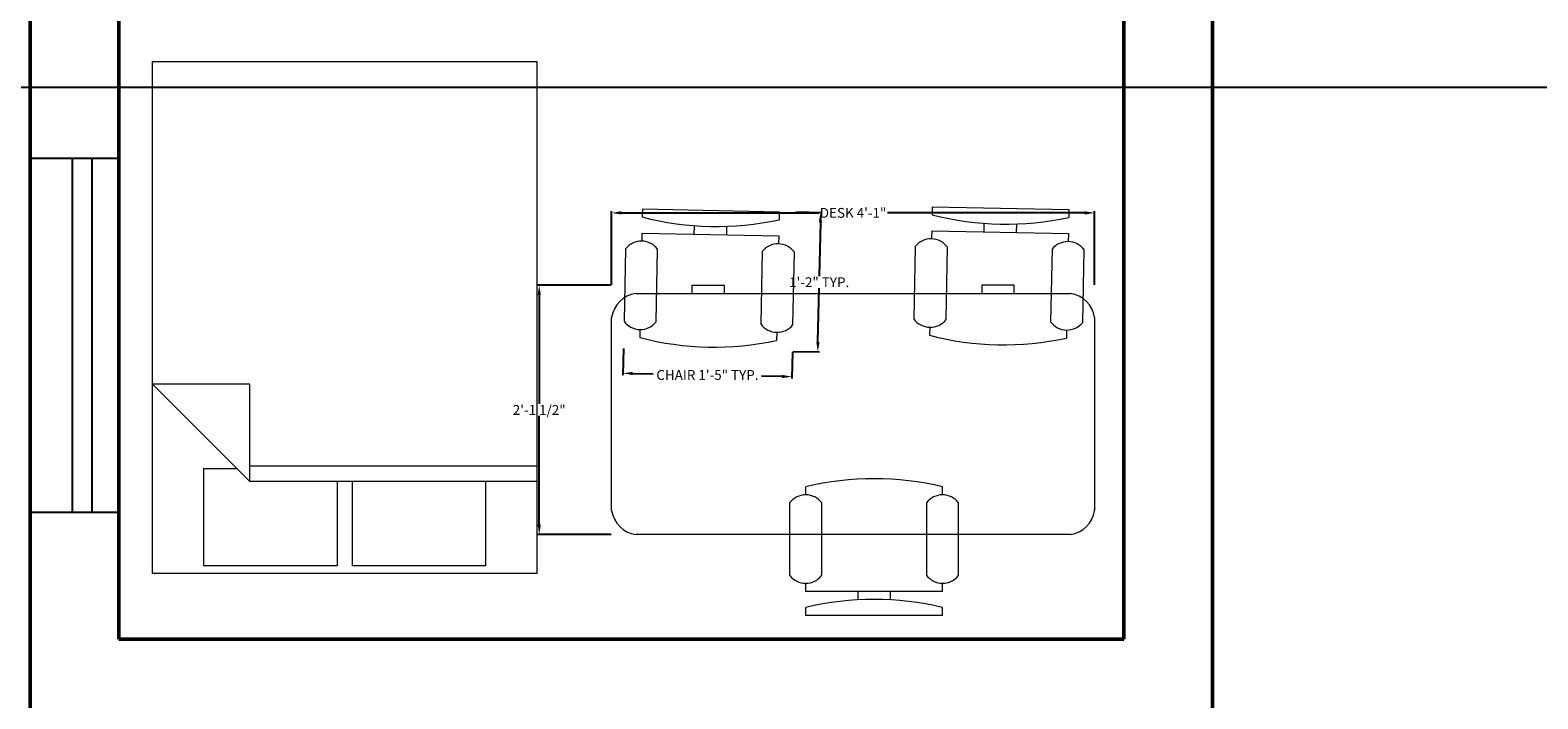
# Model space of a CAD drawing. Units: inches. Extents: x -364 to 705, y -52 to 1250.
# Tile 9 of 34: x 29 to 182, y 580 to 648. Entities that reach past the tile are written whole.
import ezdxf

# ---------------------------------------------------------------- set-up
doc = ezdxf.new("R2010")
doc.units = ezdxf.units.IN
doc.header["$MEASUREMENT"] = 0
for name, color, linetype, lineweight in [('A-ANNO-DIMS', 4, 'Continuous', 18), ('A-FURN', 8, 'Continuous', 18), ('A-GLAZ', 4, 'Continuous', 25), ('A-WALL', 41, 'Continuous', 50)]:
    doc.layers.add(name, color=color, linetype=linetype, lineweight=lineweight)
doc.styles.get("Standard").update_dxf_attribs({"font": 'arial.ttf'})
doc.dimstyles.get("Standard").update_dxf_attribs({"dimtxt": 1, "dimasz": 1, "dimexe": 0.18, "dimexo": 0.0625, "dimgap": 0.09, "dimtad": 0, "dimtih": 1, "dimtoh": 1, "dimdec": 0, "dimzin": 0, "dimdsep": 46, "dimlunit": 3, "dimtxsty": 'Standard', "dimcen": 0.09, "dimadec": 0, "dimazin": 0, "dimtfac": 1, "dimtdec": 0, "dimtofl": 0, "dimtmove": 0, "dimatfit": 3, "dimfxl": 1, "dimtolj": 1, "dimtzin": 0, "dimarcsym": 0})

# ---------------------------------------------------------------- blocks, each defined once
blk = doc.blocks.new('Chair - Desk')
for p, q in [((-8.5, 0), (-8.5, -1)), ((-8.5, 0), (8.5, 0)), ((8.5, 0), (8.5, -1)), ((-8.5, -3), (-8.5, -4)), ((-8.5, -3), (8.5, -3)), ((-2, -3), (-2, -1.9355)), ((2, -1.9576), (2, -3)), ((8.5, -3), (8.5, -4)), ((-10.5, -5), (-10.5, -14)), ((-6.5, -14), (-6.5, -5)), ((6.5, -5), (6.5, -14)), ((10.5, -14), (10.5, -5)), ((-8.5, -15), (-8.5, -16)), ((8.5, -15), (8.5, -16))]:
    blk.add_line(p, q)
for centre, radius, start, end in [((0, 34.625), 36.625, 256.5803, 283.4197), ((-8.5, -6.5), 2.5, 36.8699, 143.1301), ((8.5, -6.5), 2.5, 36.8699, 143.1301), ((-8.5, -12.5), 2.5, 216.8699, 323.1301), ((8.5, -12.5), 2.5, 216.8699, 323.1301), ((0, 19.625), 36.625, 256.5803, 283.4197)]:
    blk.add_arc(centre, radius, start, end)
blk = doc.blocks.new('Desk - 30 x 60 in.')
for p, q in [((-26.999995, 0), (26.999995, 0)), ((-29.999995, -27), (-29.999995, -3)), ((29.999995, -3), (29.999995, -27)), ((26.999995, -30), (-26.999995, -30)), ((-20.000005, -30), (-20.000005, -31)), ((-20.000005, -31), (-16.000005, -31)), ((-16.000005, -31), (-16.000005, -30)), ((15.999995, -31), (15.999995, -30)), ((19.999995, -31), (15.999995, -31)), ((19.999995, -30), (19.999995, -31))]:
    blk.add_line(p, q)
for centre, start, end in [((-26.499995, -3.5), 98.1301, 171.8699), ((26.499995, -3.5), 8.130102, 81.8699), ((-26.499995, -26.5), 188.1301, 261.8699), ((26.499995, -26.5), 278.1301, 351.8699)]:
    blk.add_arc(centre, 3.535534, start, end)
blk = doc.blocks.new('Bed - Queen')
for p, q in [((0, -80.00003), (0, 0)), ((0, 0), (59.99999, 0)), ((59.99999, 0), (59.99999, -80.00003)), ((7.99999, -1.2), (28.79998, -1.2)), ((7.99999, -14.4), (7.99999, -1.2)), ((28.79998, -1.2), (28.79998, -14.4)), ((31.19999, -1.2), (51.99999, -1.2)), ((31.19999, -14.4), (31.19999, -1.2)), ((51.99999, -1.2), (51.99999, -16.4)), ((0, -14.4), (44.8, -14.4)), ((59.99999, -29.6), (44.8, -14.4)), ((44.8, -14.4), (44.8, -29.6)), ((51.99999, -16.4), (46.79936, -16.4)), ((44.8, -16.8), (0, -16.8)), ((44.8, -29.6), (59.99999, -29.6)), ((59.99999, -80.00003), (0, -80.00003))]:
    blk.add_line(p, q)
blk = doc.blocks.new('*D19')
at = {"layer": 'A-ANNO-DIMS', "color": 0, "lineweight": -2, "transparency": 16777216}
for p, q in [((28.52, 986.11), (-248.33, 986.11)), ((-248.15, 985.11), (-248.15, 574.22)), ((-248.15, 149.87), (-248.15, 560.77)), ((28.52, 148.87), (-248.33, 148.87))]:
    blk.add_line(p, q, dxfattribs=at)
at = {"layer": 'A-ANNO-DIMS', "color": 0, "transparency": 16777216}
for points in [[(-248.32, 985.11), (-247.99, 985.11), (-248.15, 986.11)], [(-248.32, 149.87), (-247.99, 149.87), (-248.15, 148.87)]]:
    blk.add_solid(points, dxfattribs=at)
at = {"layer": 'Defpoints', "color": 0, "transparency": 16777216}
for p in [(28.58, 986.11), (-248.15, 148.87), (28.58, 148.87)]:
    blk.add_point(p, dxfattribs=at)
at = {"layer": 'A-ANNO-DIMS', "color": 0, "transparency": 16777216, "insert": (-248.15, 567.49), "char_height": 1, "attachment_point": 5}
blk.add_mtext('\\A1;{\\H13x;69\'-9"}', dxfattribs=at)
blk = doc.blocks.new('*D31')
at = {"layer": 'A-ANNO-DIMS', "color": 0, "lineweight": -2, "transparency": 16777216}
for p, q in [((37.52, 706.11), (-205.07, 706.11)), ((-204.89, 705.11), (-204.89, 648.34)), ((-204.89, 578.11), (-204.89, 634.89)), ((37.52, 577.11), (-205.07, 577.11))]:
    blk.add_line(p, q, dxfattribs=at)
at = {"layer": 'A-ANNO-DIMS', "color": 0, "transparency": 16777216}
for points in [[(-205.06, 705.11), (-204.73, 705.11), (-204.89, 706.11)], [(-205.06, 578.11), (-204.73, 578.11), (-204.89, 577.11)]]:
    blk.add_solid(points, dxfattribs=at)
at = {"layer": 'Defpoints', "color": 0, "transparency": 16777216}
for p in [(37.58, 706.11), (-204.89, 577.11), (37.58, 577.11)]:
    blk.add_point(p, dxfattribs=at)
at = {"layer": 'A-ANNO-DIMS', "color": 0, "transparency": 16777216, "insert": (-204.89, 641.61), "char_height": 1, "attachment_point": 5}
blk.add_mtext('\\A1;{\\H13x;10\'-9"}', dxfattribs=at)
blk = doc.blocks.new('*D42')
at = {"layer": 'A-ANNO-DIMS', "color": 0, "lineweight": -2, "transparency": 16777216}
for p, q in [((88.79, 615.6), (88.73, 612.91)), ((105.93, 615.26), (105.88, 612.57)), ((89.74, 613.07), (91.81, 613.03)), ((104.88, 612.77), (102.81, 612.81))]:
    blk.add_line(p, q, dxfattribs=at)
at = {"layer": 'A-ANNO-DIMS', "color": 0, "transparency": 16777216}
for points in [[(89.74, 613.24), (89.73, 612.91), (88.74, 613.09)], [(104.89, 612.93), (104.88, 612.6), (105.88, 612.75)]]:
    blk.add_solid(points, dxfattribs=at)
at = {"layer": 'Defpoints', "color": 0, "transparency": 16777216}
for p in [(88.79, 615.67), (105.94, 615.32), (105.88, 612.75)]:
    blk.add_point(p, dxfattribs=at)
at = {"layer": 'A-ANNO-DIMS', "color": 0, "transparency": 16777216, "insert": (97.31, 612.92), "char_height": 1, "attachment_point": 5}
blk.add_mtext('\\A1;CHAIR 1\'-5" TYP.', dxfattribs=at)
blk = doc.blocks.new('*D43')
at = {"layer": 'A-ANNO-DIMS', "color": 0, "lineweight": -2, "transparency": 16777216}
for p, q in [((106.28, 629.47), (108.97, 629.42)), ((108.77, 628.42), (108.66, 622.94)), ((108.53, 616.27), (108.64, 621.75)), ((106, 615.32), (108.69, 615.26))]:
    blk.add_line(p, q, dxfattribs=at)
at = {"layer": 'A-ANNO-DIMS', "color": 0, "transparency": 16777216}
for points in [[(108.61, 628.42), (108.94, 628.42), (108.79, 629.42)], [(108.36, 616.27), (108.69, 616.26), (108.51, 615.27)]]:
    blk.add_solid(points, dxfattribs=at)
at = {"layer": 'Defpoints', "color": 0, "transparency": 16777216}
for p in [(106.22, 629.47), (108.79, 629.42), (105.94, 615.32)]:
    blk.add_point(p, dxfattribs=at)
at = {"layer": 'A-ANNO-DIMS', "color": 0, "transparency": 16777216, "insert": (108.65, 622.34), "char_height": 1, "attachment_point": 5}
blk.add_mtext('\\A1;1\'-2" TYP.', dxfattribs=at)
blk = doc.blocks.new('*D54')
at = {"layer": 'A-ANNO-DIMS', "color": 0, "lineweight": -2, "transparency": 16777216}
for p, q in [((87.59, 622.09), (87.59, 629.56)), ((88.59, 629.38), (108.6, 629.38)), ((135.59, 629.38), (115.58, 629.38)), ((136.59, 622.09), (136.59, 629.56))]:
    blk.add_line(p, q, dxfattribs=at)
at = {"layer": 'A-ANNO-DIMS', "color": 0, "transparency": 16777216}
for points in [[(88.59, 629.55), (88.59, 629.21), (87.59, 629.38)], [(135.59, 629.55), (135.59, 629.21), (136.59, 629.38)]]:
    blk.add_solid(points, dxfattribs=at)
at = {"layer": 'Defpoints', "color": 0, "transparency": 16777216}
for p in [(87.59, 629.38), (87.59, 622.03), (136.59, 622.03)]:
    blk.add_point(p, dxfattribs=at)
at = {"layer": 'A-ANNO-DIMS', "color": 0, "transparency": 16777216, "insert": (112.09, 629.38), "char_height": 1, "attachment_point": 5}
blk.add_mtext('\\A1;DESK 4\'-1"', dxfattribs=at)
blk = doc.blocks.new('*D55')
at = {"layer": 'A-ANNO-DIMS', "color": 0, "lineweight": -2, "transparency": 16777216}
for p, q in [((87.53, 622.03), (80.06, 622.03)), ((80.24, 621.03), (80.24, 609.98)), ((80.24, 597.71), (80.24, 608.76)), ((87.53, 596.71), (80.06, 596.71))]:
    blk.add_line(p, q, dxfattribs=at)
at = {"layer": 'A-ANNO-DIMS', "color": 0, "transparency": 16777216}
for points in [[(80.08, 621.03), (80.41, 621.03), (80.24, 622.03)], [(80.08, 597.71), (80.41, 597.71), (80.24, 596.71)]]:
    blk.add_solid(points, dxfattribs=at)
at = {"layer": 'Defpoints', "color": 0, "transparency": 16777216}
for p in [(87.59, 622.03), (80.24, 596.71), (87.59, 596.71)]:
    blk.add_point(p, dxfattribs=at)
at = {"layer": 'A-ANNO-DIMS', "color": 0, "transparency": 16777216, "insert": (80.24, 609.37), "char_height": 1, "attachment_point": 5}
blk.add_mtext('\\A1;2\'-1 1/2"', dxfattribs=at)
blk = doc.blocks.new('*D98')
at = {"layer": 'A-ANNO-DIMS', "color": 0, "lineweight": -2, "transparency": 16777216}
for p, q in [((358.52, 642.11), (-126.85, 642.11)), ((-126.67, 641.11), (-126.67, 582.72)), ((-126.67, 523.11), (-126.67, 581.51)), ((358.52, 522.11), (-126.85, 522.11))]:
    blk.add_line(p, q, dxfattribs=at)
at = {"layer": 'A-ANNO-DIMS', "color": 0, "transparency": 16777216}
for points in [[(-126.84, 641.11), (-126.5, 641.11), (-126.67, 642.11)], [(-126.84, 523.11), (-126.5, 523.11), (-126.67, 522.11)]]:
    blk.add_solid(points, dxfattribs=at)
at = {"layer": 'Defpoints', "color": 0, "transparency": 16777216}
for p in [(-126.67, 642.11), (358.58, 642.11), (358.58, 522.11)]:
    blk.add_point(p, dxfattribs=at)
at = {"layer": 'A-ANNO-DIMS', "color": 0, "transparency": 16777216, "insert": (-126.67, 582.11), "char_height": 1, "attachment_point": 5}
blk.add_mtext('\\A1;10\'-0"', dxfattribs=at)

msp = doc.modelspace()

# ---------------------------------------------------------------- linework, layer by layer
at = {"layer": 'A-GLAZ'}
for p, q in [((32.85, 634.94), (32.85, 598.94)), ((34.85, 634.94), (34.85, 598.94))]:
    msp.add_line(p, q, dxfattribs=at)
msp.add_lwpolyline([(37.58, 634.94), (37.58, 598.94), (28.58, 598.94), (28.58, 634.94)], close=True, dxfattribs=at)
at = {"layer": 'A-WALL'}
for p, q in [((28.58, 11.11), (28.58, 986.11)), ((37.58, 586.11), (37.58, 835.11)), ((139.58, 586.11), (139.58, 676.98)), ((148.58, 571.14), (148.58, 676.98)), ((139.58, 586.11), (37.58, 586.11))]:
    msp.add_line(p, q, dxfattribs=at)

# ---------------------------------------------------------------- block references
at = {"layer": 'A-FURN'}
for name, p, xscale, yscale, zscale, rotation in [('Bed - Queen', (80, 592.76), 0.6500148169160638, 0.6500148169160638, 0.6500148169160638, 180), ('Chair - Desk', (97.65, 629.64), 0.8166422968664236, 0.8166422968664236, 0.8166422968664236, 358.8399543093713), ('Chair - Desk', (127.06, 629.87), 0.8166422968664236, 0.8166422968664236, 0.8166422968664236, 358.8399543093713), ('Desk - 30 x 60 in.', (112.09, 596.71), 0.8166422968664236, 0.8166422968664236, 0.8166422968664236, 180), ('Chair - Desk', (114.23, 588.5), 0.8166422968664236, 0.8166422968664236, 0.8166422968664236, 180)]:
    msp.add_blockref(name, p, dxfattribs=dict(at, xscale=xscale, yscale=yscale, zscale=zscale, rotation=rotation))

# ---------------------------------------------------------------- dimensions: what is measured, and where the dimension line sits
at = {"layer": 'A-ANNO-DIMS'}
for base, p1, p2, angle, text, override, picture, middle in [((-248.15, 148.87), (28.58, 986.11), (28.58, 148.87), 90, '{\\H13x;<>}', {"dimclrd": 0, "dimclre": 0, "dimclrt": 0}, '*D19', (-248.15, 567.49)), ((-204.89, 577.11), (37.58, 706.11), (37.58, 577.11), 90, '{\\H13x;<>}', {"dimclrd": 0, "dimclre": 0, "dimclrt": 0}, '*D31', (-204.89, 641.61)), ((87.59, 629.38), (136.59, 622.03), (87.59, 622.03), 180, 'DESK <>', {"dimdec": 1, "dimlfac": 1, "dimrnd": 0, "dimzin": 1, "dimdsep": 46, "dimlunit": 4, "dimfrac": 2}, '*D54', (112.09, 629.38)), ((108.79, 629.42), (105.94, 615.32), (106.22, 629.47), 88.84, '<> TYP.', {"dimdec": 1, "dimlfac": 1, "dimrnd": 0, "dimzin": 1, "dimdsep": 46, "dimlunit": 4, "dimfrac": 2}, '*D43', (108.65, 622.34)), ((105.8838, 612.7467), (88.7899, 615.6658), (105.9359, 615.3186), 358.84, 'CHAIR <> TYP.', {"dimdec": 1, "dimlfac": 1, "dimrnd": 0, "dimzin": 1, "dimdsep": 46, "dimlunit": 4, "dimfrac": 2}, '*D42', (97.3108, 612.9203))]:
    dim = msp.add_linear_dim(base=base, p1=p1, p2=p2, angle=angle, text=text, dimstyle='Standard', override=override, dxfattribs=at)
    dim.commit()
    dim.dimension.update_dxf_attribs({"geometry": picture, "text_midpoint": middle})
for base, p1, p2, angle, picture, middle in [((-126.67, 642.11), (358.58, 522.11), (358.58, 642.11), 90, '*D98', (-126.67, 582.11)), ((80.24, 596.71), (87.59, 622.03), (87.59, 596.71), 270, '*D55', (80.24, 609.37))]:
    dim = msp.add_linear_dim(base=base, p1=p1, p2=p2, angle=angle, dimstyle='Standard', override={"dimdec": 1, "dimlfac": 1, "dimrnd": 0, "dimzin": 1, "dimdsep": 46, "dimlunit": 4, "dimfrac": 2}, dxfattribs=at)
    dim.commit()
    dim.dimension.update_dxf_attribs({"geometry": picture, "text_midpoint": middle})

doc.saveas('drawing.dxf')
